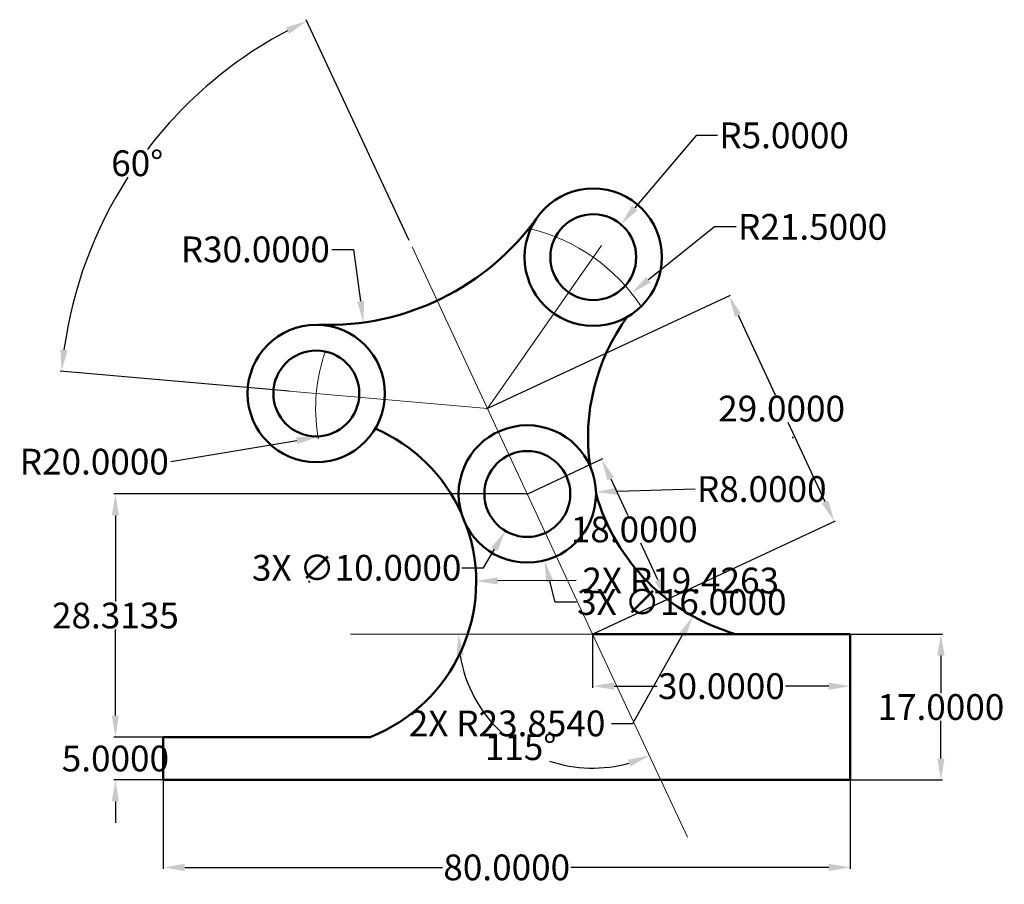
# Model space of a CAD drawing. Units: inches. Extents: x 444 to 559, y 213 to 313.
import ezdxf

# ---------------------------------------------------------------- set-up
doc = ezdxf.new("R2010")
doc.units = ezdxf.units.IN
doc.header["$MEASUREMENT"] = 0
doc.linetypes.add('CENTER', pattern=[50.8, 31.75, -6.35, 6.35, -6.35])
for name, color, linetype, lineweight in [('M-CNTR', 4, 'CENTER', 18), ('M-CONS', 8, 'Continuous', 13), ('M-DIMS', 2, 'Continuous', 25), ('M-OUTL', 7, 'Continuous', 50)]:
    doc.layers.add(name, color=color, linetype=linetype, lineweight=lineweight)
doc.styles.get("Standard").update_dxf_attribs({"font": 'arial.ttf'})
doc.dimstyles.get("Standard").update_dxf_attribs({"dimtxt": 3, "dimasz": 2.5, "dimexe": 0.18, "dimexo": 0.0625, "dimgap": 0.09, "dimtad": 0, "dimtih": 1, "dimtoh": 1, "dimdec": 4, "dimzin": 0, "dimdsep": 46, "dimtxsty": 'Standard', "dimcen": 0.09, "dimadec": 0, "dimazin": 0, "dimtfac": 1, "dimtdec": 4, "dimtofl": 0, "dimtmove": 0, "dimatfit": 3, "dimfxl": 1, "dimtolj": 1, "dimtzin": 0, "dimarcsym": 0})

# ---------------------------------------------------------------- blocks, each defined once
blk = doc.blocks.new('*D1')
at = {"layer": 'Defpoints', "color": 0, "transparency": 16777216}
for p in [(503.16, 258.24), (511.15, 258.47)]:
    blk.add_point(p, dxfattribs=at)
at = {"layer": 'M-DIMS', "color": 0, "lineweight": -2, "transparency": 16777216}
for p, q in [((503.07, 258.24), (503.25, 258.24)), ((503.16, 258.15), (503.16, 258.33)), ((522.72, 258.81), (513.65, 258.54))]:
    blk.add_line(p, q, dxfattribs=at)
at = {"layer": 'M-DIMS', "color": 0, "transparency": 16777216}
blk.add_solid([(513.64, 258.96), (513.66, 258.13), (511.15, 258.47)], dxfattribs=at)
at = {"layer": 'M-DIMS', "color": 0, "transparency": 16777216, "insert": (530.46, 258.81), "char_height": 3, "attachment_point": 5}
blk.add_mtext('\\A1;R8.0000', dxfattribs=at)
blk = doc.blocks.new('*D2')
at = {"layer": 'Defpoints', "color": 0, "transparency": 16777216}
for p in [(498.51, 268.2), (478.78, 264.89)]:
    blk.add_point(p, dxfattribs=at)
at = {"layer": 'M-DIMS', "color": 0, "lineweight": -2, "transparency": 16777216}
for p, q in [((498.42, 268.2), (498.6, 268.2)), ((498.51, 268.11), (498.51, 268.29)), ((461.64, 262), (476.32, 264.47))]:
    blk.add_line(p, q, dxfattribs=at)
blk.add_arc((498.51, 268.2), 20, 189.5406, 190.0673, dxfattribs=at)
at = {"layer": 'M-DIMS', "color": 0, "transparency": 16777216}
blk.add_solid([(476.25, 264.88), (476.39, 264.06), (478.78, 264.89)], dxfattribs=at)
at = {"layer": 'M-DIMS', "color": 0, "transparency": 16777216, "insert": (452.73, 262), "char_height": 3, "attachment_point": 5}
blk.add_mtext('\\A1;R20.0000', dxfattribs=at)
blk = doc.blocks.new('*D3')
at = {"layer": 'Defpoints', "color": 0, "transparency": 16777216}
for p in [(515.3, 281.63), (498.51, 268.2)]:
    blk.add_point(p, dxfattribs=at)
at = {"layer": 'M-DIMS', "color": 0, "lineweight": -2, "transparency": 16777216}
for p, q in [((524.97, 289.35), (517.26, 283.19)), ((527.47, 289.35), (524.97, 289.35)), ((498.42, 268.2), (498.6, 268.2)), ((498.51, 268.11), (498.51, 268.29))]:
    blk.add_line(p, q, dxfattribs=at)
at = {"layer": 'M-DIMS', "color": 0, "transparency": 16777216}
blk.add_solid([(517, 283.51), (517.52, 282.86), (515.3, 281.63)], dxfattribs=at)
at = {"layer": 'M-DIMS', "color": 0, "transparency": 16777216, "insert": (536.38, 289.35), "char_height": 3, "attachment_point": 5}
blk.add_mtext('\\A1;R21.5000', dxfattribs=at)
blk = doc.blocks.new('*D4')
at = {"layer": 'Defpoints', "color": 0, "transparency": 16777216}
for p in [(479.93, 307.92), (484.09, 278.21)]:
    blk.add_point(p, dxfattribs=at)
at = {"layer": 'M-DIMS', "color": 0, "lineweight": -2, "transparency": 16777216}
for p, q in [((480.4, 286.73), (482.9, 286.73)), ((482.9, 286.73), (483.74, 280.69))]:
    blk.add_line(p, q, dxfattribs=at)
at = {"layer": 'M-DIMS', "color": 0, "transparency": 16777216}
blk.add_solid([(484.15, 280.75), (483.33, 280.63), (484.09, 278.21)], dxfattribs=at)
at = {"layer": 'M-DIMS', "color": 0, "transparency": 16777216, "insert": (471.48, 286.73), "char_height": 3, "attachment_point": 5}
blk.add_mtext('\\A1;R30.0000', dxfattribs=at)
blk = doc.blocks.new('*D5')
at = {"layer": 'Defpoints', "color": 0, "transparency": 16777216}
for p in [(460.76, 224.92), (540.76, 224.92), (540.76, 214.74)]:
    blk.add_point(p, dxfattribs=at)
at = {"layer": 'M-DIMS', "color": 0, "lineweight": -2, "transparency": 16777216}
for p, q in [((460.76, 224.86), (460.76, 214.56)), ((540.76, 224.86), (540.76, 214.56)), ((463.26, 214.74), (493.28, 214.74)), ((538.26, 214.74), (508.24, 214.74))]:
    blk.add_line(p, q, dxfattribs=at)
at = {"layer": 'M-DIMS', "color": 0, "transparency": 16777216}
for points in [[(463.26, 215.15), (463.26, 214.32), (460.76, 214.74)], [(538.26, 215.15), (538.26, 214.32), (540.76, 214.74)]]:
    blk.add_solid(points, dxfattribs=at)
at = {"layer": 'M-DIMS', "color": 0, "transparency": 16777216, "insert": (500.76, 214.74), "char_height": 3, "attachment_point": 5}
blk.add_mtext('\\A1;80.0000', dxfattribs=at)
blk = doc.blocks.new('*D6')
at = {"layer": 'Defpoints', "color": 0, "transparency": 16777216}
for p in [(463.31, 303.4), (489.42, 287.69), (475.43, 270.22), (498.51, 268.2), (503.16, 258.24)]:
    blk.add_point(p, dxfattribs=at)
at = {"layer": 'M-DIMS', "color": 0, "lineweight": -2, "transparency": 16777216}
for p, q in [((489.39, 287.75), (477.39, 313.48)), ((475.37, 270.23), (448.74, 272.56))]:
    blk.add_line(p, q, dxfattribs=at)
for start, end in [(117.8778, 142.688), (147.2484, 172.1222)]:
    blk.add_arc((498.51, 268.2), 49.78, start, end, dxfattribs=at)
at = {"layer": 'M-DIMS', "color": 0, "transparency": 16777216}
for points in [[(475.05, 312.58), (475.42, 311.83), (477.47, 313.32)], [(449.61, 274.98), (448.78, 275.07), (448.92, 272.54)]]:
    blk.add_solid(points, dxfattribs=at)
at = {"layer": 'M-DIMS', "color": 0, "transparency": 16777216, "insert": (457.73, 296.76), "char_height": 3, "attachment_point": 5}
blk.add_mtext('\\A1;60°', dxfattribs=at)
blk = doc.blocks.new('*D7')
at = {"layer": 'Defpoints', "color": 0, "transparency": 16777216}
for p in [(514.06, 289.64), (510.84, 285.82)]:
    blk.add_point(p, dxfattribs=at)
at = {"layer": 'M-DIMS', "color": 0, "lineweight": -2, "transparency": 16777216}
for p, q in [((522.81, 300.01), (515.67, 291.55)), ((525.31, 300.01), (522.81, 300.01)), ((510.75, 285.82), (510.93, 285.82)), ((510.84, 285.73), (510.84, 285.91))]:
    blk.add_line(p, q, dxfattribs=at)
at = {"layer": 'M-DIMS', "color": 0, "transparency": 16777216}
blk.add_solid([(515.36, 291.82), (515.99, 291.28), (514.06, 289.64)], dxfattribs=at)
at = {"layer": 'M-DIMS', "color": 0, "transparency": 16777216, "insert": (533.06, 300.01), "char_height": 3, "attachment_point": 5}
blk.add_mtext('\\A1;R5.0000', dxfattribs=at)
blk = doc.blocks.new('*D8')
at = {"layer": 'Defpoints', "color": 0, "transparency": 16777216}
for p in [(510.76, 241.92), (540.76, 241.92), (540.76, 235.85)]:
    blk.add_point(p, dxfattribs=at)
at = {"layer": 'M-DIMS', "color": 0, "lineweight": -2, "transparency": 16777216}
for p, q in [((510.76, 241.86), (510.76, 235.67)), ((540.76, 241.86), (540.76, 235.67)), ((513.26, 235.85), (518.29, 235.85)), ((538.26, 235.85), (533.24, 235.85))]:
    blk.add_line(p, q, dxfattribs=at)
at = {"layer": 'M-DIMS', "color": 0, "transparency": 16777216}
for points in [[(513.26, 236.27), (513.26, 235.43), (510.76, 235.85)], [(538.26, 236.27), (538.26, 235.43), (540.76, 235.85)]]:
    blk.add_solid(points, dxfattribs=at)
at = {"layer": 'M-DIMS', "color": 0, "transparency": 16777216, "insert": (525.76, 235.85), "char_height": 3, "attachment_point": 5}
blk.add_mtext('\\A1;30.0000', dxfattribs=at)
blk = doc.blocks.new('*D9')
at = {"layer": 'Defpoints', "color": 0, "transparency": 16777216}
for p in [(511.81, 262.27), (503.16, 258.24), (510.76, 241.92)]:
    blk.add_point(p, dxfattribs=at)
at = {"layer": 'M-DIMS', "color": 0, "lineweight": -2, "transparency": 16777216}
for p, q in [((503.21, 258.26), (511.97, 262.35)), ((512.87, 260.01), (514.86, 255.74)), ((518.36, 248.22), (516.37, 252.49)), ((510.82, 241.95), (519.58, 246.03))]:
    blk.add_line(p, q, dxfattribs=at)
at = {"layer": 'M-DIMS', "color": 0, "transparency": 16777216}
for points in [[(513.25, 260.18), (512.49, 259.83), (511.81, 262.27)], [(518.74, 248.4), (517.98, 248.05), (519.42, 245.96)]]:
    blk.add_solid(points, dxfattribs=at)
at = {"layer": 'M-DIMS', "color": 0, "transparency": 16777216, "insert": (515.61, 254.11), "char_height": 3, "attachment_point": 5}
blk.add_mtext('\\A1;18.0000', dxfattribs=at)
blk = doc.blocks.new('*D10')
at = {"layer": 'Defpoints', "color": 0, "transparency": 16777216}
for p in [(526.64, 281.32), (498.51, 268.2), (510.76, 241.92)]:
    blk.add_point(p, dxfattribs=at)
at = {"layer": 'M-DIMS', "color": 0, "lineweight": -2, "transparency": 16777216}
for p, q in [((498.56, 268.23), (526.8, 281.4)), ((527.7, 279.06), (532.01, 269.8)), ((537.84, 257.31), (533.52, 266.56)), ((510.82, 241.95), (539.06, 255.12))]:
    blk.add_line(p, q, dxfattribs=at)
at = {"layer": 'M-DIMS', "color": 0, "transparency": 16777216}
for points in [[(528.07, 279.23), (527.32, 278.88), (526.64, 281.32)], [(538.22, 257.48), (537.46, 257.13), (538.9, 255.04)]]:
    blk.add_solid(points, dxfattribs=at)
at = {"layer": 'M-DIMS', "color": 0, "transparency": 16777216, "insert": (532.77, 268.18), "char_height": 3, "attachment_point": 5}
blk.add_mtext('\\A1;29.0000', dxfattribs=at)
blk = doc.blocks.new('*D11')
at = {"layer": 'Defpoints', "color": 0, "transparency": 16777216}
for p in [(540.76, 241.92), (551.32, 241.92), (540.76, 224.92)]:
    blk.add_point(p, dxfattribs=at)
at = {"layer": 'M-DIMS', "color": 0, "lineweight": -2, "transparency": 16777216}
for p, q in [((540.83, 241.92), (551.5, 241.92)), ((551.32, 239.42), (551.32, 235.04)), ((551.32, 227.42), (551.32, 231.8)), ((540.83, 224.92), (551.5, 224.92))]:
    blk.add_line(p, q, dxfattribs=at)
at = {"layer": 'M-DIMS', "color": 0, "transparency": 16777216}
for points in [[(550.9, 239.42), (551.74, 239.42), (551.32, 241.92)], [(550.9, 227.42), (551.74, 227.42), (551.32, 224.92)]]:
    blk.add_solid(points, dxfattribs=at)
at = {"layer": 'M-DIMS', "color": 0, "transparency": 16777216, "insert": (551.32, 233.42), "char_height": 3, "attachment_point": 5}
blk.add_mtext('\\A1;17.0000', dxfattribs=at)
blk = doc.blocks.new('*D12')
at = {"layer": 'Defpoints', "color": 0, "transparency": 16777216}
for p in [(482.56, 241.92), (510.76, 241.92), (510.76, 241.92), (498.51, 232.23), (521.8, 218.26)]:
    blk.add_point(p, dxfattribs=at)
at = {"layer": 'M-DIMS', "color": 0, "lineweight": -2, "transparency": 16777216}
for start, end in [(189.1774, 227.6972), (251.2955, 285.8226)]:
    blk.add_arc((510.76, 241.92), 15.62, start, end, dxfattribs=at)
at = {"layer": 'M-DIMS', "color": 0, "transparency": 16777216}
for points in [[(494.92, 239.4), (495.75, 239.46), (495.14, 241.92)], [(514.88, 227.28), (515.17, 226.5), (517.37, 227.76)]]:
    blk.add_solid(points, dxfattribs=at)
at = {"layer": 'M-DIMS', "color": 0, "transparency": 16777216, "insert": (502.37, 228.74), "char_height": 3, "attachment_point": 5}
blk.add_mtext('\\A1;115°', dxfattribs=at)
blk = doc.blocks.new('PIVOT-LOBE-OD16-BORE10')
for radius in [8, 5]:
    blk.add_circle((8, 8), radius)
blk = doc.blocks.new('*D14')
at = {"layer": 'Defpoints', "color": 0, "transparency": 16777216}
for p in [(455.19, 229.92), (460.76, 229.92), (460.76, 224.92)]:
    blk.add_point(p, dxfattribs=at)
at = {"layer": 'M-DIMS', "color": 0, "lineweight": -2, "transparency": 16777216}
for p, q in [((455.19, 232.42), (455.19, 234.92)), ((460.7, 229.92), (455.01, 229.92)), ((460.7, 224.92), (455.01, 224.92)), ((455.19, 222.42), (455.19, 219.92))]:
    blk.add_line(p, q, dxfattribs=at)
at = {"layer": 'M-DIMS', "color": 0, "transparency": 16777216}
for points in [[(454.77, 232.42), (455.6, 232.42), (455.19, 229.92)], [(454.77, 222.42), (455.6, 222.42), (455.19, 224.92)]]:
    blk.add_solid(points, dxfattribs=at)
at = {"layer": 'M-DIMS', "color": 0, "transparency": 16777216, "insert": (455.19, 227.42), "char_height": 3, "attachment_point": 5}
blk.add_mtext('\\A1;5.0000', dxfattribs=at)
blk = doc.blocks.new('*D15')
at = {"layer": 'Defpoints', "color": 0, "transparency": 16777216}
for p in [(455.19, 258.24), (503.16, 258.24), (460.76, 229.92)]:
    blk.add_point(p, dxfattribs=at)
at = {"layer": 'M-DIMS', "color": 0, "lineweight": -2, "transparency": 16777216}
for p, q in [((503.09, 258.24), (455.01, 258.24)), ((455.19, 255.74), (455.19, 245.7)), ((455.19, 232.42), (455.19, 242.46)), ((460.7, 229.92), (455.01, 229.92))]:
    blk.add_line(p, q, dxfattribs=at)
at = {"layer": 'M-DIMS', "color": 0, "transparency": 16777216}
for points in [[(454.77, 255.74), (455.6, 255.74), (455.19, 258.24)], [(454.77, 232.42), (455.6, 232.42), (455.19, 229.92)]]:
    blk.add_solid(points, dxfattribs=at)
at = {"layer": 'M-DIMS', "color": 0, "transparency": 16777216, "insert": (455.19, 244.08), "char_height": 3, "attachment_point": 5}
blk.add_mtext('\\A1;28.3135', dxfattribs=at)
blk = doc.blocks.new('*D16')
at = {"layer": 'Defpoints', "color": 0, "transparency": 16777216}
for p in [(501.16, 265.98), (505.15, 250.49)]:
    blk.add_point(p, dxfattribs=at)
at = {"layer": 'M-DIMS', "color": 0, "lineweight": -2, "transparency": 16777216}
for p, q in [((503.07, 258.24), (503.25, 258.24)), ((503.16, 258.15), (503.16, 258.33)), ((506.4, 245.65), (505.77, 248.07)), ((508.9, 245.65), (506.4, 245.65))]:
    blk.add_line(p, q, dxfattribs=at)
at = {"layer": 'M-DIMS', "color": 0, "transparency": 16777216}
blk.add_solid([(506.18, 248.17), (505.37, 247.96), (505.15, 250.49)], dxfattribs=at)
at = {"layer": 'M-DIMS', "color": 0, "transparency": 16777216, "insert": (521.15, 245.65), "char_height": 3, "attachment_point": 5}
blk.add_mtext('\\A1;3X ∅16.0000', dxfattribs=at)
blk = doc.blocks.new('*D17')
at = {"layer": 'Defpoints', "color": 0, "transparency": 16777216}
for p in [(505.71, 262.53), (500.6, 253.94)]:
    blk.add_point(p, dxfattribs=at)
at = {"layer": 'M-DIMS', "color": 0, "lineweight": -2, "transparency": 16777216}
for p, q in [((503.07, 258.24), (503.25, 258.24)), ((503.16, 258.15), (503.16, 258.33)), ((498.04, 249.64), (499.32, 251.79)), ((495.54, 249.64), (498.04, 249.64))]:
    blk.add_line(p, q, dxfattribs=at)
at = {"layer": 'M-DIMS', "color": 0, "transparency": 16777216}
blk.add_solid([(498.96, 252), (499.68, 251.58), (500.6, 253.94)], dxfattribs=at)
at = {"layer": 'M-DIMS', "color": 0, "transparency": 16777216, "insert": (483.29, 249.64), "char_height": 3, "attachment_point": 5}
blk.add_mtext('\\A1;3X ∅10.0000', dxfattribs=at)
blk = doc.blocks.new('*D18')
at = {"layer": 'Defpoints', "color": 0, "transparency": 16777216}
for p in [(534.08, 264.82), (522.44, 244)]:
    blk.add_point(p, dxfattribs=at)
at = {"layer": 'M-DIMS', "color": 0, "lineweight": -2, "transparency": 16777216}
for p, q in [((534.08, 264.73), (534.08, 264.91)), ((533.99, 264.82), (534.17, 264.82)), ((515.46, 231.51), (521.22, 241.82)), ((512.96, 231.51), (515.46, 231.51))]:
    blk.add_line(p, q, dxfattribs=at)
at = {"layer": 'M-DIMS', "color": 0, "transparency": 16777216}
blk.add_solid([(520.86, 242.02), (521.59, 241.61), (522.44, 244)], dxfattribs=at)
at = {"layer": 'M-DIMS', "color": 0, "transparency": 16777216, "insert": (500.8, 231.51), "char_height": 3, "attachment_point": 5}
blk.add_mtext('\\A1;2X R23.8540', dxfattribs=at)
blk = doc.blocks.new('*D19')
at = {"layer": 'Defpoints', "color": 0, "transparency": 16777216}
for p in [(477.77, 248.01), (497.2, 248.1)]:
    blk.add_point(p, dxfattribs=at)
at = {"layer": 'M-DIMS', "color": 0, "lineweight": -2, "transparency": 16777216}
for p, q in [((477.68, 248.01), (477.86, 248.01)), ((477.77, 247.92), (477.77, 248.1)), ((508.85, 248.15), (499.7, 248.11))]:
    blk.add_line(p, q, dxfattribs=at)
at = {"layer": 'M-DIMS', "color": 0, "transparency": 16777216}
blk.add_solid([(499.7, 248.53), (499.7, 247.69), (497.2, 248.1)], dxfattribs=at)
at = {"layer": 'M-DIMS', "color": 0, "transparency": 16777216, "insert": (521.02, 248.15), "char_height": 3, "attachment_point": 5}
blk.add_mtext('\\A1;2X R19.4263', dxfattribs=at)

msp = doc.modelspace()

# ---------------------------------------------------------------- linework, layer by layer
at = {"layer": 'M-CNTR'}
for p, q in [((503.15576, 258.23551), (489.42066, 287.69051)), ((498.50696, 268.20489), (511.79151, 287.17719)), ((498.50696, 268.20489), (475.43419, 270.2235)), ((510.76289, 241.92197), (503.15576, 258.23551)), ((510.76289, 241.92197), (521.79707, 218.25908))]:
    msp.add_line(p, q, dxfattribs=at)
at = {"layer": 'M-CONS'}
msp.add_line((510.76289, 241.92197), (482.55785, 241.92197), dxfattribs=at)
for radius, start, end in [(21.5, 33.5556952, 76.4443048), (20, 160.6384884, 189.3615116)]:
    msp.add_arc((498.50696, 268.20489), radius, start, end, dxfattribs=at)
at = {"layer": 'M-OUTL'}
for p, q in [((540.76289, 241.92197), (510.76289, 241.92197)), ((540.76289, 224.92197), (540.76289, 241.92197)), ((460.76289, 224.92197), (460.76289, 229.92197)), ((460.76289, 229.92197), (484.85905, 229.92197)), ((460.76289, 224.92197), (540.76289, 224.92197))]:
    msp.add_line(p, q, dxfattribs=at)
for centre, radius, start, end in [((479.93153, 307.92407), 30, 267.9663732, 324.4245858), ((534.08256, 264.82145), 23.85399, 143.9252186, 188.0161989), ((477.77308, 248.00976), 19.42625, 24.397165, 66.7057935), ((534.08256, 264.82145), 23.85399, 196.0272147, 253.7367796), ((477.77308, 248.00976), 19.42625, 291.3929802, 19.4882241)]:
    msp.add_arc(centre, radius, start, end, dxfattribs=at)

# ---------------------------------------------------------------- block references
for p in [(502.83909, 277.81715), (470.58331, 261.9485), (495.156, 250.236)]:
    msp.add_blockref('PIVOT-LOBE-OD16-BORE10', p, dxfattribs=at)

# ---------------------------------------------------------------- dimensions: what is measured, and where the dimension line sits
at = {"layer": 'M-DIMS'}
for base, line1, line2, picture, middle in [((463.30767, 303.40418), ((503.15576, 258.23551), (489.42066, 287.69051)), ((498.50696, 268.20489), (475.43419, 270.2235)), '*D6', (457.73013, 296.75713)), ((498.50682, 232.23112), ((510.76289, 241.92197), (482.55785, 241.92197)), ((510.76289, 241.92197), (521.79707, 218.25908)), '*D12', (502.36787, 228.74443))]:
    dim = msp.add_angular_dim_2l(base=base, line1=line1, line2=line2, dimstyle='Standard', override={"dimclrd": 0, "dimclre": 0, "dimclrt": 0}, dxfattribs=at)
    dim.commit()
    dim.dimension.update_dxf_attribs({"geometry": picture, "text_midpoint": middle})
for center, mpoint, picture, middle in [((479.93153, 307.92407), (484.08715, 278.21329), '*D4', (471.48362, 286.72514)), ((510.83885, 285.81666), (514.06232, 289.63886), '*D7', (533.06059, 300.01491)), ((498.50696, 268.20489), (515.30281, 281.62687), '*D3', (536.3834, 289.35249)), ((498.50696, 268.20489), (478.78423, 264.88616), '*D2', (461.64037, 262.00137)), ((503.15576, 258.23551), (511.15231, 258.47036), '*D1', (522.7172, 258.81002))]:
    dim = msp.add_radius_dim(center=center, mpoint=mpoint, dimstyle='Standard', override={"dimclrd": 0, "dimclre": 0, "dimclrt": 0}, dxfattribs=at)
    dim.commit()
    dim.dimension.update_dxf_attribs({"geometry": picture, "text_midpoint": middle, "dimtype": 164})
for p1, p2, distance, picture, middle in [((510.76289, 241.92197), (498.50696, 268.20489), -31.0415, '*D10', (532.76808, 268.18214)), ((510.76289, 241.92197), (503.15576, 258.23551), -9.55019, '*D9', (515.61474, 254.11482)), ((540.76289, 224.92197), (540.76289, 241.92197), -10.55662, '*D11', (551.31951, 233.42197))]:
    dim = msp.add_aligned_dim(p1=p1, p2=p2, distance=distance, dimstyle='Standard', override={"dimclrd": 0, "dimclre": 0, "dimclrt": 0}, dxfattribs=at)
    dim.commit()
    dim.dimension.update_dxf_attribs({"geometry": picture, "text_midpoint": middle})
for center, mpoint, picture, middle in [((534.08256, 264.82145), (522.44383, 243.99951), '*D18', (500.79897, 231.50635)), ((477.773081, 248.009758), (497.199123, 248.099996), '*D19', (508.854748, 248.154139))]:
    dim = msp.add_radius_dim(center=center, mpoint=mpoint, text='2X <>', dimstyle='Standard', override={"dimdec": 4, "dimlfac": 1, "dimrnd": 0, "dimzin": 0, "dimdsep": 46, "dimlunit": 2}, dxfattribs=at)
    dim.commit()
    dim.dimension.update_dxf_attribs({"geometry": picture, "text_midpoint": middle, "dimtype": 164})
dim = msp.add_diameter_dim_2p(p1=(501.16104, 265.98284), p2=(505.15047, 250.48818), text='3X <>', dimstyle='Standard', override={"dimdec": 4, "dimlfac": 1, "dimrnd": 0, "dimzin": 0, "dimdsep": 46, "dimlunit": 2}, dxfattribs=at)
dim.commit()
dim.dimension.update_dxf_attribs({"geometry": '*D16', "text_midpoint": (521.14883, 245.64609)})
dim = msp.add_diameter_dim_2p(p1=(505.71237, 262.53245), p2=(500.59914, 253.93856), text='3X <>', dimstyle='Standard', override={"dimdec": 4, "dimlfac": 1, "dimrnd": 0, "dimzin": 0, "dimdsep": 46, "dimlunit": 2}, dxfattribs=at)
dim.commit()
dim.dimension.update_dxf_attribs({"geometry": '*D17', "text_midpoint": (483.29087, 249.64162), "dimtype": 163})
for base, p1, p2, picture, middle in [((455.18789, 258.23551), (460.76289, 229.92197), (503.15576, 258.23551), '*D15', (455.18789, 244.07874)), ((455.18789, 229.92197), (460.76289, 224.92197), (460.76289, 229.92197), '*D14', (455.18789, 227.42197))]:
    dim = msp.add_linear_dim(base=base, p1=p1, p2=p2, angle=90, dimstyle='Standard', override={"dimdec": 4, "dimlfac": 1, "dimrnd": 0, "dimzin": 0, "dimdsep": 46, "dimlunit": 2}, dxfattribs=at)
    dim.commit()
    dim.dimension.update_dxf_attribs({"geometry": picture, "text_midpoint": middle})
for base, p1, p2, picture, middle in [((540.76289, 235.85037), (510.76289, 241.92197), (540.76289, 241.92197), '*D8', (525.76289, 235.85037)), ((540.76289, 214.73598), (460.76289, 224.92197), (540.76289, 224.92197), '*D5', (500.76289, 214.73598))]:
    dim = msp.add_linear_dim(base=base, p1=p1, p2=p2, dimstyle='Standard', override={"dimclrd": 0, "dimclre": 0, "dimclrt": 0}, dxfattribs=at)
    dim.commit()
    dim.dimension.update_dxf_attribs({"geometry": picture, "text_midpoint": middle})

doc.saveas('drawing.dxf')
